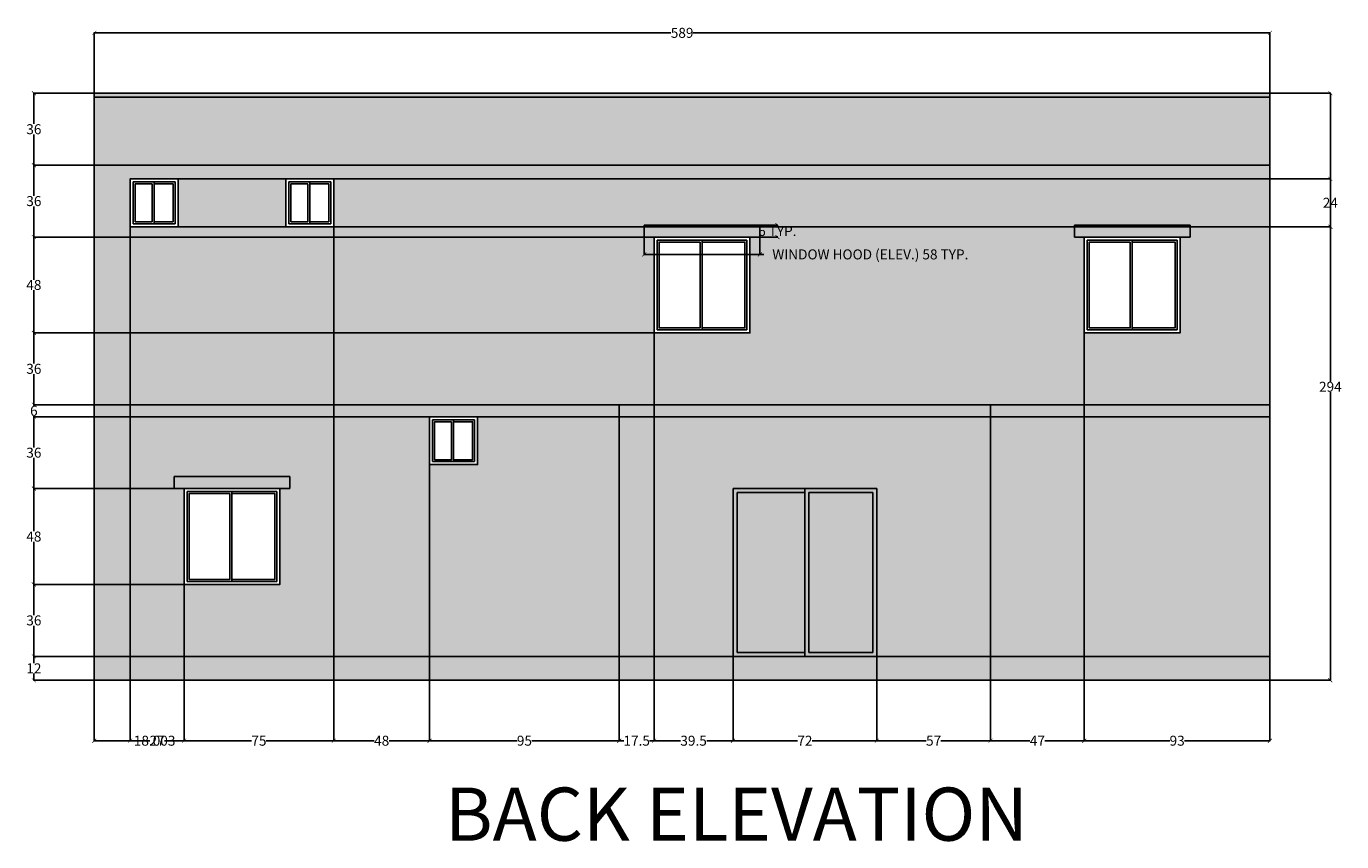
# Model space of a CAD drawing. Units: inches. Extents: x 1455 to 5994, y -182 to 2370.
# Tile 8 of 8: x 5335 to 5994, y -182 to 227. Entities that reach past the tile are written whole.
import ezdxf

# ---------------------------------------------------------------- set-up
doc = ezdxf.new("R2010")
doc.units = ezdxf.units.IN
doc.header["$MEASUREMENT"] = 0
for name, color, linetype, lineweight in [('A-ANNO-DIMS', 2, 'Continuous', 18), ('A-ANNO-TEXT', 7, 'Continuous', 25), ('A-ELEV', 7, 'Continuous', 25), ('A-ELEV-PATT', 8, 'Continuous', 13)]:
    doc.layers.add(name, color=color, linetype=linetype, lineweight=lineweight)
doc.styles.get("Standard").update_dxf_attribs({"font": 'arial.ttf'})
doc.dimstyles.get("Standard").update_dxf_attribs({"dimtxt": 5, "dimasz": 2, "dimexe": 0.18, "dimexo": 0.0625, "dimgap": 0.09, "dimtad": 0, "dimtih": 1, "dimtoh": 1, "dimdec": 1, "dimzin": 0, "dimdsep": 46, "dimlunit": 3, "dimtxsty": 'Standard', "dimblk": 'ARCHTICK', "dimcen": 0.09, "dimadec": 0, "dimazin": 0, "dimtfac": 1, "dimtdec": 1, "dimtofl": 0, "dimtmove": 0, "dimatfit": 3, "dimfxl": 1, "dimtolj": 1, "dimtzin": 0, "dimarcsym": 0})

# ---------------------------------------------------------------- blocks, each defined once
blk = doc.blocks.new('*U8')
for p, q in [((1.5, 1.5), (1.5, 46.5)), ((1.5, 46.5), (24, 46.5)), ((24, 1.5), (24, 46.5)), ((24, 46.5), (46.5, 46.5)), ((46.5, 46.5), (46.5, 1.5)), ((24, 1.5), (1.5, 1.5)), ((46.5, 1.5), (24, 1.5))]:
    blk.add_line(p, q)
blk.add_lwpolyline([(0, 0), (0, 48), (48, 48), (48, 0)], close=True)
for points in [[(23, 45.5), (23, 2.5), (2.5, 2.5), (2.5, 45.5), (23, 45.5)], [(24, 45.5), (45.5, 45.5), (45.5, 2.5), (24, 2.5)]]:
    blk.add_lwpolyline(points)
blk = doc.blocks.new('*U13')
for p, q in [((1.5, 1.5), (1.5, 22.5)), ((1.5, 22.5), (12, 22.5)), ((12, 1.5), (12, 22.5)), ((12, 22.5), (22.5, 22.5)), ((22.5, 22.5), (22.5, 1.5)), ((12, 1.5), (1.5, 1.5)), ((22.5, 1.5), (12, 1.5))]:
    blk.add_line(p, q)
blk.add_lwpolyline([(0, 0), (0, 24), (24, 24), (24, 0)], close=True)
for points in [[(11, 21.5), (11, 2.5), (2.5, 2.5), (2.5, 21.5), (11, 21.5)], [(12, 21.5), (21.5, 21.5), (21.5, 2.5), (12, 2.5)]]:
    blk.add_lwpolyline(points)
blk = doc.blocks.new('WIN-HOOD-ELEV')
for p, q in [((0, 0), (0, 6)), ((0, 6), (58, 6)), ((58, 0), (58, 6)), ((5, 0), (0, 0)), ((53, 0), (58, 0))]:
    blk.add_line(p, q)
blk = doc.blocks.new('_ArchTick')
at = {"color": 0, "linetype": 'ByBlock', "const_width": 0.15}
blk.add_lwpolyline([(-0.5, -0.5), (0.5, 0.5)], dxfattribs=at)
blk = doc.blocks.new('*D33')
at = {"layer": 'A-ANNO-DIMS', "color": 0, "lineweight": -2, "transparency": 16777216}
for p, q in [((5644.62, 121.03), (5644.62, 112.22)), ((5702.62, 121.03), (5702.62, 112.22)), ((5644.62, 112.4), (5702.62, 112.4)), ((5702.62, 112.4), (5704.62, 112.4))]:
    blk.add_line(p, q, dxfattribs=at)
at = {"layer": 'Defpoints', "color": 0, "lineweight": 25, "transparency": 16777216}
for p in [(5644.62, 121.1), (5702.62, 121.1), (5702.62, 112.4)]:
    blk.add_point(p, dxfattribs=at)
at = {"layer": 'A-ANNO-DIMS', "color": 0, "lineweight": -2, "transparency": 16777216, "xscale": 2, "yscale": 2, "zscale": 2, "rotation": 180}
blk.add_blockref('_ArchTick', (5644.62, 112.4), dxfattribs=at)
at = {"layer": 'A-ANNO-DIMS', "color": 0, "lineweight": -2, "transparency": 16777216, "xscale": 2, "yscale": 2, "zscale": 2}
blk.add_blockref('_ArchTick', (5702.62, 112.4), dxfattribs=at)
at = {"layer": 'A-ANNO-DIMS', "color": 0, "transparency": 16777216, "insert": (5757.92, 112.4), "char_height": 5, "attachment_point": 5}
blk.add_mtext('\\A1;WINDOW HOOD (ELEV.) 58 TYP.', dxfattribs=at)
blk = doc.blocks.new('*D34')
at = {"layer": 'A-ANNO-DIMS', "color": 0, "lineweight": -2, "transparency": 16777216}
for p, q in [((5702.68, 127.1), (5711.5, 127.1)), ((5711.32, 127.1), (5711.32, 126.74)), ((5702.68, 121.1), (5711.5, 121.1)), ((5711.32, 121.1), (5711.32, 121.45))]:
    blk.add_line(p, q, dxfattribs=at)
at = {"layer": 'Defpoints', "color": 0, "lineweight": 25, "transparency": 16777216}
for p in [(5702.62, 127.1), (5711.32, 127.1), (5702.62, 121.1)]:
    blk.add_point(p, dxfattribs=at)
at = {"layer": 'A-ANNO-DIMS', "color": 0, "lineweight": -2, "transparency": 16777216, "xscale": 2, "yscale": 2, "zscale": 2}
for p, rotation in [((5711.32, 127.1), 90), ((5711.32, 121.1), 270)]:
    blk.add_blockref('_ArchTick', p, dxfattribs=dict(at, rotation=rotation))
at = {"layer": 'A-ANNO-DIMS', "color": 0, "transparency": 16777216, "insert": (5711.32, 124.1), "char_height": 5, "attachment_point": 5}
blk.add_mtext('\\A1;6 TYP.', dxfattribs=at)
blk = doc.blocks.new('*D117')
at = {"layer": 'A-ANNO-DIMS', "color": 0, "lineweight": -2, "transparency": 16777216}
for p, q in [((5369.12, 193.16), (5369.12, 223.53)), ((5369.12, 223.35), (5658, 223.35)), ((5958.12, 223.35), (5669.24, 223.35)), ((5958.12, 193.16), (5958.12, 223.53))]:
    blk.add_line(p, q, dxfattribs=at)
at = {"layer": 'Defpoints', "color": 0, "lineweight": 25, "transparency": 16777216}
for p in [(5958.12, 223.35), (5369.12, 193.1), (5958.12, 193.1)]:
    blk.add_point(p, dxfattribs=at)
at = {"layer": 'A-ANNO-DIMS', "color": 0, "lineweight": -2, "transparency": 16777216, "xscale": 2, "yscale": 2, "zscale": 2, "rotation": 180}
blk.add_blockref('_ArchTick', (5369.12, 223.35), dxfattribs=at)
at = {"layer": 'A-ANNO-DIMS', "color": 0, "lineweight": -2, "transparency": 16777216, "xscale": 2, "yscale": 2, "zscale": 2}
blk.add_blockref('_ArchTick', (5958.12, 223.35), dxfattribs=at)
at = {"layer": 'A-ANNO-DIMS', "color": 0, "transparency": 16777216, "insert": (5663.62, 223.35), "char_height": 5, "attachment_point": 5}
blk.add_mtext('\\A1;589', dxfattribs=at)
blk = doc.blocks.new('*D118')
at = {"layer": 'A-ANNO-DIMS', "color": 0, "lineweight": -2, "transparency": 16777216}
for p, q in [((5958.18, 193.1), (5988.55, 193.1)), ((5988.37, 193.1), (5988.37, 48.74)), ((5988.37, -100.9), (5988.37, 43.45)), ((5958.18, -100.9), (5988.55, -100.9))]:
    blk.add_line(p, q, dxfattribs=at)
at = {"layer": 'Defpoints', "color": 0, "lineweight": 25, "transparency": 16777216}
for p in [(5958.12, 193.1), (5988.37, 193.1), (5958.12, -100.9)]:
    blk.add_point(p, dxfattribs=at)
at = {"layer": 'A-ANNO-DIMS', "color": 0, "lineweight": -2, "transparency": 16777216, "xscale": 2, "yscale": 2, "zscale": 2}
for p, rotation in [((5988.37, 193.1), 90), ((5988.37, -100.9), 270)]:
    blk.add_blockref('_ArchTick', p, dxfattribs=dict(at, rotation=rotation))
at = {"layer": 'A-ANNO-DIMS', "color": 0, "transparency": 16777216, "insert": (5988.37, 46.1), "char_height": 5, "attachment_point": 5}
blk.add_mtext('\\A1;294', dxfattribs=at)
blk = doc.blocks.new('*D119')
at = {"layer": 'A-ANNO-DIMS', "color": 0, "lineweight": -2, "transparency": 16777216}
for p, q in [((5387.12, 126.2), (5387.12, -131.33)), ((5369.12, -100.97), (5369.12, -131.33)), ((5369.12, -131.15), (5387.12, -131.15)), ((5387.12, -131.15), (5389.12, -131.15))]:
    blk.add_line(p, q, dxfattribs=at)
at = {"layer": 'Defpoints', "color": 0, "lineweight": 25, "transparency": 16777216}
for p in [(5387.12, 126.26), (5369.12, -100.9), (5387.12, -131.15)]:
    blk.add_point(p, dxfattribs=at)
at = {"layer": 'A-ANNO-DIMS', "color": 0, "lineweight": -2, "transparency": 16777216, "xscale": 2, "yscale": 2, "zscale": 2, "rotation": 180}
blk.add_blockref('_ArchTick', (5369.12, -131.15), dxfattribs=at)
at = {"layer": 'A-ANNO-DIMS', "color": 0, "lineweight": -2, "transparency": 16777216, "xscale": 2, "yscale": 2, "zscale": 2}
blk.add_blockref('_ArchTick', (5387.12, -131.15), dxfattribs=at)
at = {"layer": 'A-ANNO-DIMS', "color": 0, "transparency": 16777216, "insert": (5399.36, -131.15), "char_height": 5, "attachment_point": 5}
blk.add_mtext('\\A1;18.003', dxfattribs=at)
blk = doc.blocks.new('*D120')
at = {"layer": 'A-ANNO-DIMS', "color": 0, "lineweight": -2, "transparency": 16777216}
for p, q in [((5387.12, 126.2), (5387.12, -131.33)), ((5414.12, -52.97), (5414.12, -131.33)), ((5387.12, -131.15), (5396.91, -131.15)), ((5414.12, -131.15), (5404.34, -131.15))]:
    blk.add_line(p, q, dxfattribs=at)
at = {"layer": 'Defpoints', "color": 0, "lineweight": 25, "transparency": 16777216}
for p in [(5387.12, 126.26), (5414.12, -52.9), (5414.12, -131.15)]:
    blk.add_point(p, dxfattribs=at)
at = {"layer": 'A-ANNO-DIMS', "color": 0, "lineweight": -2, "transparency": 16777216, "xscale": 2, "yscale": 2, "zscale": 2, "rotation": 180}
blk.add_blockref('_ArchTick', (5387.12, -131.15), dxfattribs=at)
at = {"layer": 'A-ANNO-DIMS', "color": 0, "lineweight": -2, "transparency": 16777216, "xscale": 2, "yscale": 2, "zscale": 2}
blk.add_blockref('_ArchTick', (5414.12, -131.15), dxfattribs=at)
at = {"layer": 'A-ANNO-DIMS', "color": 0, "transparency": 16777216, "insert": (5400.62, -131.15), "char_height": 5, "attachment_point": 5}
blk.add_mtext('\\A1;27', dxfattribs=at)
blk = doc.blocks.new('*D121')
at = {"layer": 'A-ANNO-DIMS', "color": 0, "lineweight": -2, "transparency": 16777216}
for p, q in [((5489.12, 126.2), (5489.12, -131.33)), ((5414.12, -52.97), (5414.12, -131.33)), ((5414.12, -131.15), (5447.95, -131.15)), ((5489.12, -131.15), (5455.29, -131.15))]:
    blk.add_line(p, q, dxfattribs=at)
at = {"layer": 'Defpoints', "color": 0, "lineweight": 25, "transparency": 16777216}
for p in [(5489.12, 126.26), (5414.12, -52.9), (5489.12, -131.15)]:
    blk.add_point(p, dxfattribs=at)
at = {"layer": 'A-ANNO-DIMS', "color": 0, "lineweight": -2, "transparency": 16777216, "xscale": 2, "yscale": 2, "zscale": 2, "rotation": 180}
blk.add_blockref('_ArchTick', (5414.12, -131.15), dxfattribs=at)
at = {"layer": 'A-ANNO-DIMS', "color": 0, "lineweight": -2, "transparency": 16777216, "xscale": 2, "yscale": 2, "zscale": 2}
blk.add_blockref('_ArchTick', (5489.12, -131.15), dxfattribs=at)
at = {"layer": 'A-ANNO-DIMS', "color": 0, "transparency": 16777216, "insert": (5451.62, -131.15), "char_height": 5, "attachment_point": 5}
blk.add_mtext('\\A1;75', dxfattribs=at)
blk = doc.blocks.new('*D122')
at = {"layer": 'A-ANNO-DIMS', "color": 0, "lineweight": -2, "transparency": 16777216}
for p, q in [((5489.12, 126.2), (5489.12, -131.33)), ((5537.12, 7.03), (5537.12, -131.33)), ((5489.12, -131.15), (5509.34, -131.15)), ((5537.12, -131.15), (5516.9, -131.15))]:
    blk.add_line(p, q, dxfattribs=at)
at = {"layer": 'Defpoints', "color": 0, "lineweight": 25, "transparency": 16777216}
for p in [(5489.12, 126.26), (5537.12, 7.1), (5537.12, -131.15)]:
    blk.add_point(p, dxfattribs=at)
at = {"layer": 'A-ANNO-DIMS', "color": 0, "lineweight": -2, "transparency": 16777216, "xscale": 2, "yscale": 2, "zscale": 2, "rotation": 180}
blk.add_blockref('_ArchTick', (5489.12, -131.15), dxfattribs=at)
at = {"layer": 'A-ANNO-DIMS', "color": 0, "lineweight": -2, "transparency": 16777216, "xscale": 2, "yscale": 2, "zscale": 2}
blk.add_blockref('_ArchTick', (5537.12, -131.15), dxfattribs=at)
at = {"layer": 'A-ANNO-DIMS', "color": 0, "transparency": 16777216, "insert": (5513.12, -131.15), "char_height": 5, "attachment_point": 5}
blk.add_mtext('\\A1;48', dxfattribs=at)
blk = doc.blocks.new('*D123')
at = {"layer": 'A-ANNO-DIMS', "color": 0, "lineweight": -2, "transparency": 16777216}
for p, q in [((5537.12, 7.03), (5537.12, -131.33)), ((5632.12, -88.97), (5632.12, -131.33)), ((5537.12, -131.15), (5580.93, -131.15)), ((5632.12, -131.15), (5588.31, -131.15))]:
    blk.add_line(p, q, dxfattribs=at)
at = {"layer": 'Defpoints', "color": 0, "lineweight": 25, "transparency": 16777216}
for p in [(5537.12, 7.1), (5632.12, -88.9), (5632.12, -131.15)]:
    blk.add_point(p, dxfattribs=at)
at = {"layer": 'A-ANNO-DIMS', "color": 0, "lineweight": -2, "transparency": 16777216, "xscale": 2, "yscale": 2, "zscale": 2, "rotation": 180}
blk.add_blockref('_ArchTick', (5537.12, -131.15), dxfattribs=at)
at = {"layer": 'A-ANNO-DIMS', "color": 0, "lineweight": -2, "transparency": 16777216, "xscale": 2, "yscale": 2, "zscale": 2}
blk.add_blockref('_ArchTick', (5632.12, -131.15), dxfattribs=at)
at = {"layer": 'A-ANNO-DIMS', "color": 0, "transparency": 16777216, "insert": (5584.62, -131.15), "char_height": 5, "attachment_point": 5}
blk.add_mtext('\\A1;95', dxfattribs=at)
blk = doc.blocks.new('*D124')
at = {"layer": 'A-ANNO-DIMS', "color": 0, "lineweight": -2, "transparency": 16777216}
for p, q in [((5649.62, 73.03), (5649.62, -131.33)), ((5632.12, -88.97), (5632.12, -131.33)), ((5632.12, -131.15), (5634.5, -131.15)), ((5649.62, -131.15), (5647.24, -131.15))]:
    blk.add_line(p, q, dxfattribs=at)
at = {"layer": 'Defpoints', "color": 0, "lineweight": 25, "transparency": 16777216}
for p in [(5649.62, 73.1), (5632.12, -88.9), (5649.62, -131.15)]:
    blk.add_point(p, dxfattribs=at)
at = {"layer": 'A-ANNO-DIMS', "color": 0, "lineweight": -2, "transparency": 16777216, "xscale": 2, "yscale": 2, "zscale": 2, "rotation": 180}
blk.add_blockref('_ArchTick', (5632.12, -131.15), dxfattribs=at)
at = {"layer": 'A-ANNO-DIMS', "color": 0, "lineweight": -2, "transparency": 16777216, "xscale": 2, "yscale": 2, "zscale": 2}
blk.add_blockref('_ArchTick', (5649.62, -131.15), dxfattribs=at)
at = {"layer": 'A-ANNO-DIMS', "color": 0, "transparency": 16777216, "insert": (5640.87, -131.15), "char_height": 5, "attachment_point": 5}
blk.add_mtext('\\A1;17.5', dxfattribs=at)
blk = doc.blocks.new('*D125')
at = {"layer": 'A-ANNO-DIMS', "color": 0, "lineweight": -2, "transparency": 16777216}
for p, q in [((5649.62, 73.03), (5649.62, -131.33)), ((5689.12, -88.97), (5689.12, -131.33)), ((5649.62, -131.15), (5662.77, -131.15)), ((5689.12, -131.15), (5675.97, -131.15))]:
    blk.add_line(p, q, dxfattribs=at)
at = {"layer": 'Defpoints', "color": 0, "lineweight": 25, "transparency": 16777216}
for p in [(5649.62, 73.1), (5689.12, -88.9), (5689.12, -131.15)]:
    blk.add_point(p, dxfattribs=at)
at = {"layer": 'A-ANNO-DIMS', "color": 0, "lineweight": -2, "transparency": 16777216, "xscale": 2, "yscale": 2, "zscale": 2, "rotation": 180}
blk.add_blockref('_ArchTick', (5649.62, -131.15), dxfattribs=at)
at = {"layer": 'A-ANNO-DIMS', "color": 0, "lineweight": -2, "transparency": 16777216, "xscale": 2, "yscale": 2, "zscale": 2}
blk.add_blockref('_ArchTick', (5689.12, -131.15), dxfattribs=at)
at = {"layer": 'A-ANNO-DIMS', "color": 0, "transparency": 16777216, "insert": (5669.37, -131.15), "char_height": 5, "attachment_point": 5}
blk.add_mtext('\\A1;39.5', dxfattribs=at)
blk = doc.blocks.new('*D126')
at = {"layer": 'A-ANNO-DIMS', "color": 0, "lineweight": -2, "transparency": 16777216}
for p, q in [((5689.12, -88.97), (5689.12, -131.33)), ((5761.12, -88.97), (5761.12, -131.33)), ((5689.12, -131.15), (5721.49, -131.15)), ((5761.12, -131.15), (5728.75, -131.15))]:
    blk.add_line(p, q, dxfattribs=at)
at = {"layer": 'Defpoints', "color": 0, "lineweight": 25, "transparency": 16777216}
for p in [(5689.12, -88.9), (5761.12, -88.9), (5761.12, -131.15)]:
    blk.add_point(p, dxfattribs=at)
at = {"layer": 'A-ANNO-DIMS', "color": 0, "lineweight": -2, "transparency": 16777216, "xscale": 2, "yscale": 2, "zscale": 2, "rotation": 180}
blk.add_blockref('_ArchTick', (5689.12, -131.15), dxfattribs=at)
at = {"layer": 'A-ANNO-DIMS', "color": 0, "lineweight": -2, "transparency": 16777216, "xscale": 2, "yscale": 2, "zscale": 2}
blk.add_blockref('_ArchTick', (5761.12, -131.15), dxfattribs=at)
at = {"layer": 'A-ANNO-DIMS', "color": 0, "transparency": 16777216, "insert": (5725.12, -131.15), "char_height": 5, "attachment_point": 5}
blk.add_mtext('\\A1;72', dxfattribs=at)
blk = doc.blocks.new('*D127')
at = {"layer": 'A-ANNO-DIMS', "color": 0, "lineweight": -2, "transparency": 16777216}
for p, q in [((5761.12, -88.97), (5761.12, -131.33)), ((5818.12, -88.97), (5818.12, -131.33)), ((5761.12, -131.15), (5785.95, -131.15)), ((5818.12, -131.15), (5793.29, -131.15))]:
    blk.add_line(p, q, dxfattribs=at)
at = {"layer": 'Defpoints', "color": 0, "lineweight": 25, "transparency": 16777216}
for p in [(5761.12, -88.9), (5818.12, -88.9), (5818.12, -131.15)]:
    blk.add_point(p, dxfattribs=at)
at = {"layer": 'A-ANNO-DIMS', "color": 0, "lineweight": -2, "transparency": 16777216, "xscale": 2, "yscale": 2, "zscale": 2, "rotation": 180}
blk.add_blockref('_ArchTick', (5761.12, -131.15), dxfattribs=at)
at = {"layer": 'A-ANNO-DIMS', "color": 0, "lineweight": -2, "transparency": 16777216, "xscale": 2, "yscale": 2, "zscale": 2}
blk.add_blockref('_ArchTick', (5818.12, -131.15), dxfattribs=at)
at = {"layer": 'A-ANNO-DIMS', "color": 0, "transparency": 16777216, "insert": (5789.62, -131.15), "char_height": 5, "attachment_point": 5}
blk.add_mtext('\\A1;57', dxfattribs=at)
blk = doc.blocks.new('*D128')
at = {"layer": 'A-ANNO-DIMS', "color": 0, "lineweight": -2, "transparency": 16777216}
for p, q in [((5865.12, 73.03), (5865.12, -131.33)), ((5818.12, -88.97), (5818.12, -131.33)), ((5818.12, -131.15), (5837.85, -131.15)), ((5865.12, -131.15), (5845.39, -131.15))]:
    blk.add_line(p, q, dxfattribs=at)
at = {"layer": 'Defpoints', "color": 0, "lineweight": 25, "transparency": 16777216}
for p in [(5865.12, 73.1), (5818.12, -88.9), (5865.12, -131.15)]:
    blk.add_point(p, dxfattribs=at)
at = {"layer": 'A-ANNO-DIMS', "color": 0, "lineweight": -2, "transparency": 16777216, "xscale": 2, "yscale": 2, "zscale": 2, "rotation": 180}
blk.add_blockref('_ArchTick', (5818.12, -131.15), dxfattribs=at)
at = {"layer": 'A-ANNO-DIMS', "color": 0, "lineweight": -2, "transparency": 16777216, "xscale": 2, "yscale": 2, "zscale": 2}
blk.add_blockref('_ArchTick', (5865.12, -131.15), dxfattribs=at)
at = {"layer": 'A-ANNO-DIMS', "color": 0, "transparency": 16777216, "insert": (5841.62, -131.15), "char_height": 5, "attachment_point": 5}
blk.add_mtext('\\A1;47', dxfattribs=at)
blk = doc.blocks.new('*D129')
at = {"layer": 'A-ANNO-DIMS', "color": 0, "lineweight": -2, "transparency": 16777216}
for p, q in [((5865.12, 73.03), (5865.12, -131.33)), ((5958.12, -100.97), (5958.12, -131.33)), ((5865.12, -131.15), (5907.95, -131.15)), ((5958.12, -131.15), (5915.29, -131.15))]:
    blk.add_line(p, q, dxfattribs=at)
at = {"layer": 'Defpoints', "color": 0, "lineweight": 25, "transparency": 16777216}
for p in [(5865.12, 73.1), (5958.12, -100.9), (5958.12, -131.15)]:
    blk.add_point(p, dxfattribs=at)
at = {"layer": 'A-ANNO-DIMS', "color": 0, "lineweight": -2, "transparency": 16777216, "xscale": 2, "yscale": 2, "zscale": 2, "rotation": 180}
blk.add_blockref('_ArchTick', (5865.12, -131.15), dxfattribs=at)
at = {"layer": 'A-ANNO-DIMS', "color": 0, "lineweight": -2, "transparency": 16777216, "xscale": 2, "yscale": 2, "zscale": 2}
blk.add_blockref('_ArchTick', (5958.12, -131.15), dxfattribs=at)
at = {"layer": 'A-ANNO-DIMS', "color": 0, "transparency": 16777216, "insert": (5911.62, -131.15), "char_height": 5, "attachment_point": 5}
blk.add_mtext('\\A1;93', dxfattribs=at)
blk = doc.blocks.new('*D130')
at = {"layer": 'A-ANNO-DIMS', "color": 0, "lineweight": -2, "transparency": 16777216}
for p, q in [((5369.06, -88.9), (5338.69, -88.9)), ((5338.87, -88.9), (5338.87, -92.3)), ((5338.87, -100.9), (5338.87, -97.5)), ((5369.06, -100.9), (5338.69, -100.9))]:
    blk.add_line(p, q, dxfattribs=at)
at = {"layer": 'Defpoints', "color": 0, "lineweight": 25, "transparency": 16777216}
for p in [(5338.87, -88.9), (5369.12, -88.9), (5369.12, -100.9)]:
    blk.add_point(p, dxfattribs=at)
at = {"layer": 'A-ANNO-DIMS', "color": 0, "lineweight": -2, "transparency": 16777216, "xscale": 2, "yscale": 2, "zscale": 2}
for p, rotation in [((5338.87, -88.9), 90), ((5338.87, -100.9), 270)]:
    blk.add_blockref('_ArchTick', p, dxfattribs=dict(at, rotation=rotation))
at = {"layer": 'A-ANNO-DIMS', "color": 0, "transparency": 16777216, "insert": (5338.87, -94.9), "char_height": 5, "attachment_point": 5}
blk.add_mtext('\\A1;12', dxfattribs=at)
blk = doc.blocks.new('*D131')
at = {"layer": 'A-ANNO-DIMS', "color": 0, "lineweight": -2, "transparency": 16777216}
for p, q in [((5414.06, -52.9), (5338.69, -52.9)), ((5338.87, -52.9), (5338.87, -68.26)), ((5338.87, -88.9), (5338.87, -73.55)), ((5369.06, -88.9), (5338.69, -88.9))]:
    blk.add_line(p, q, dxfattribs=at)
at = {"layer": 'Defpoints', "color": 0, "lineweight": 25, "transparency": 16777216}
for p in [(5338.87, -52.9), (5414.12, -52.9), (5369.12, -88.9)]:
    blk.add_point(p, dxfattribs=at)
at = {"layer": 'A-ANNO-DIMS', "color": 0, "lineweight": -2, "transparency": 16777216, "xscale": 2, "yscale": 2, "zscale": 2}
for p, rotation in [((5338.87, -52.9), 90), ((5338.87, -88.9), 270)]:
    blk.add_blockref('_ArchTick', p, dxfattribs=dict(at, rotation=rotation))
at = {"layer": 'A-ANNO-DIMS', "color": 0, "transparency": 16777216, "insert": (5338.87, -70.9), "char_height": 5, "attachment_point": 5}
blk.add_mtext('\\A1;36', dxfattribs=at)
blk = doc.blocks.new('*D132')
at = {"layer": 'A-ANNO-DIMS', "color": 0, "lineweight": -2, "transparency": 16777216}
for p, q in [((5414.06, -4.9), (5338.69, -4.9)), ((5338.87, -4.9), (5338.87, -26.26)), ((5338.87, -52.9), (5338.87, -31.55)), ((5414.06, -52.9), (5338.69, -52.9))]:
    blk.add_line(p, q, dxfattribs=at)
at = {"layer": 'Defpoints', "color": 0, "lineweight": 25, "transparency": 16777216}
for p in [(5338.87, -4.9), (5414.12, -4.9), (5414.12, -52.9)]:
    blk.add_point(p, dxfattribs=at)
at = {"layer": 'A-ANNO-DIMS', "color": 0, "lineweight": -2, "transparency": 16777216, "xscale": 2, "yscale": 2, "zscale": 2}
for p, rotation in [((5338.87, -4.9), 90), ((5338.87, -52.9), 270)]:
    blk.add_blockref('_ArchTick', p, dxfattribs=dict(at, rotation=rotation))
at = {"layer": 'A-ANNO-DIMS', "color": 0, "transparency": 16777216, "insert": (5338.87, -28.9), "char_height": 5, "attachment_point": 5}
blk.add_mtext('\\A1;48', dxfattribs=at)
blk = doc.blocks.new('*D133')
at = {"layer": 'A-ANNO-DIMS', "color": 0, "lineweight": -2, "transparency": 16777216}
for p, q in [((5369.06, 31.1), (5338.69, 31.1)), ((5338.87, 31.1), (5338.87, 15.74)), ((5338.87, -4.9), (5338.87, 10.45)), ((5414.06, -4.9), (5338.69, -4.9))]:
    blk.add_line(p, q, dxfattribs=at)
at = {"layer": 'Defpoints', "color": 0, "lineweight": 25, "transparency": 16777216}
for p in [(5338.87, 31.1), (5369.12, 31.1), (5414.12, -4.9)]:
    blk.add_point(p, dxfattribs=at)
at = {"layer": 'A-ANNO-DIMS', "color": 0, "lineweight": -2, "transparency": 16777216, "xscale": 2, "yscale": 2, "zscale": 2}
for p, rotation in [((5338.87, 31.1), 90), ((5338.87, -4.9), 270)]:
    blk.add_blockref('_ArchTick', p, dxfattribs=dict(at, rotation=rotation))
at = {"layer": 'A-ANNO-DIMS', "color": 0, "transparency": 16777216, "insert": (5338.87, 13.1), "char_height": 5, "attachment_point": 5}
blk.add_mtext('\\A1;36', dxfattribs=at)
blk = doc.blocks.new('*D134')
at = {"layer": 'A-ANNO-DIMS', "color": 0, "lineweight": -2, "transparency": 16777216}
for p, q in [((5369.06, 37.1), (5338.69, 37.1)), ((5338.87, 37.1), (5338.87, 36.74)), ((5369.06, 31.1), (5338.69, 31.1)), ((5338.87, 31.1), (5338.87, 31.45))]:
    blk.add_line(p, q, dxfattribs=at)
at = {"layer": 'Defpoints', "color": 0, "lineweight": 25, "transparency": 16777216}
for p in [(5338.87, 37.1), (5369.12, 37.1), (5369.12, 31.1)]:
    blk.add_point(p, dxfattribs=at)
at = {"layer": 'A-ANNO-DIMS', "color": 0, "lineweight": -2, "transparency": 16777216, "xscale": 2, "yscale": 2, "zscale": 2}
for p, rotation in [((5338.87, 37.1), 90), ((5338.87, 31.1), 270)]:
    blk.add_blockref('_ArchTick', p, dxfattribs=dict(at, rotation=rotation))
at = {"layer": 'A-ANNO-DIMS', "color": 0, "transparency": 16777216, "insert": (5338.87, 34.1), "char_height": 5, "attachment_point": 5}
blk.add_mtext('\\A1;6', dxfattribs=at)
blk = doc.blocks.new('*D135')
at = {"layer": 'A-ANNO-DIMS', "color": 0, "lineweight": -2, "transparency": 16777216}
for p, q in [((5649.56, 73.1), (5338.69, 73.1)), ((5338.87, 73.1), (5338.87, 57.74)), ((5338.87, 37.1), (5338.87, 52.45)), ((5369.06, 37.1), (5338.69, 37.1))]:
    blk.add_line(p, q, dxfattribs=at)
at = {"layer": 'Defpoints', "color": 0, "lineweight": 25, "transparency": 16777216}
for p in [(5338.87, 73.1), (5649.62, 73.1), (5369.12, 37.1)]:
    blk.add_point(p, dxfattribs=at)
at = {"layer": 'A-ANNO-DIMS', "color": 0, "lineweight": -2, "transparency": 16777216, "xscale": 2, "yscale": 2, "zscale": 2}
for p, rotation in [((5338.87, 73.1), 90), ((5338.87, 37.1), 270)]:
    blk.add_blockref('_ArchTick', p, dxfattribs=dict(at, rotation=rotation))
at = {"layer": 'A-ANNO-DIMS', "color": 0, "transparency": 16777216, "insert": (5338.87, 55.1), "char_height": 5, "attachment_point": 5}
blk.add_mtext('\\A1;36', dxfattribs=at)
blk = doc.blocks.new('*D136')
at = {"layer": 'A-ANNO-DIMS', "color": 0, "lineweight": -2, "transparency": 16777216}
for p, q in [((5649.56, 121.1), (5338.69, 121.1)), ((5338.87, 121.1), (5338.87, 99.74)), ((5338.87, 73.1), (5338.87, 94.45)), ((5649.56, 73.1), (5338.69, 73.1))]:
    blk.add_line(p, q, dxfattribs=at)
at = {"layer": 'Defpoints', "color": 0, "lineweight": 25, "transparency": 16777216}
for p in [(5338.87, 121.1), (5649.62, 121.1), (5649.62, 73.1)]:
    blk.add_point(p, dxfattribs=at)
at = {"layer": 'A-ANNO-DIMS', "color": 0, "lineweight": -2, "transparency": 16777216, "xscale": 2, "yscale": 2, "zscale": 2}
for p, rotation in [((5338.87, 121.1), 90), ((5338.87, 73.1), 270)]:
    blk.add_blockref('_ArchTick', p, dxfattribs=dict(at, rotation=rotation))
at = {"layer": 'A-ANNO-DIMS', "color": 0, "transparency": 16777216, "insert": (5338.87, 97.1), "char_height": 5, "attachment_point": 5}
blk.add_mtext('\\A1;48', dxfattribs=at)
blk = doc.blocks.new('*D137')
at = {"layer": 'A-ANNO-DIMS', "color": 0, "lineweight": -2, "transparency": 16777216}
for p, q in [((5369.06, 157.1), (5338.69, 157.1)), ((5338.87, 157.1), (5338.87, 141.74)), ((5338.87, 121.1), (5338.87, 136.45)), ((5649.56, 121.1), (5338.69, 121.1))]:
    blk.add_line(p, q, dxfattribs=at)
at = {"layer": 'Defpoints', "color": 0, "lineweight": 25, "transparency": 16777216}
for p in [(5338.87, 157.1), (5369.12, 157.1), (5649.62, 121.1)]:
    blk.add_point(p, dxfattribs=at)
at = {"layer": 'A-ANNO-DIMS', "color": 0, "lineweight": -2, "transparency": 16777216, "xscale": 2, "yscale": 2, "zscale": 2}
for p, rotation in [((5338.87, 157.1), 90), ((5338.87, 121.1), 270)]:
    blk.add_blockref('_ArchTick', p, dxfattribs=dict(at, rotation=rotation))
at = {"layer": 'A-ANNO-DIMS', "color": 0, "transparency": 16777216, "insert": (5338.87, 139.1), "char_height": 5, "attachment_point": 5}
blk.add_mtext('\\A1;36', dxfattribs=at)
blk = doc.blocks.new('*D138')
at = {"layer": 'A-ANNO-DIMS', "color": 0, "lineweight": -2, "transparency": 16777216}
for p, q in [((5369.06, 193.1), (5338.69, 193.1)), ((5338.87, 193.1), (5338.87, 177.74)), ((5338.87, 157.1), (5338.87, 172.45)), ((5369.06, 157.1), (5338.69, 157.1))]:
    blk.add_line(p, q, dxfattribs=at)
at = {"layer": 'Defpoints', "color": 0, "lineweight": 25, "transparency": 16777216}
for p in [(5338.87, 193.1), (5369.12, 193.1), (5369.12, 157.1)]:
    blk.add_point(p, dxfattribs=at)
at = {"layer": 'A-ANNO-DIMS', "color": 0, "lineweight": -2, "transparency": 16777216, "xscale": 2, "yscale": 2, "zscale": 2}
for p, rotation in [((5338.87, 193.1), 90), ((5338.87, 157.1), 270)]:
    blk.add_blockref('_ArchTick', p, dxfattribs=dict(at, rotation=rotation))
at = {"layer": 'A-ANNO-DIMS', "color": 0, "transparency": 16777216, "insert": (5338.87, 175.1), "char_height": 5, "attachment_point": 5}
blk.add_mtext('\\A1;36', dxfattribs=at)
blk = doc.blocks.new('*D139')
at = {"layer": 'A-ANNO-DIMS', "color": 0, "lineweight": -2, "transparency": 16777216}
for p, q in [((5411.19, 150.26), (5988.55, 150.26)), ((5988.37, 150.26), (5988.37, 140.86)), ((5988.37, 126.26), (5988.37, 135.66)), ((5411.19, 126.26), (5988.55, 126.26))]:
    blk.add_line(p, q, dxfattribs=at)
at = {"layer": 'Defpoints', "color": 0, "lineweight": 25, "transparency": 16777216}
for p in [(5411.12, 150.26), (5988.37, 150.26), (5411.12, 126.26)]:
    blk.add_point(p, dxfattribs=at)
at = {"layer": 'A-ANNO-DIMS', "color": 0, "lineweight": -2, "transparency": 16777216, "xscale": 2, "yscale": 2, "zscale": 2}
for p, rotation in [((5988.37, 150.26), 90), ((5988.37, 126.26), 270)]:
    blk.add_blockref('_ArchTick', p, dxfattribs=dict(at, rotation=rotation))
at = {"layer": 'A-ANNO-DIMS', "color": 0, "transparency": 16777216, "insert": (5988.37, 138.26), "char_height": 5, "attachment_point": 5}
blk.add_mtext('\\A1;24', dxfattribs=at)

msp = doc.modelspace()

# ---------------------------------------------------------------- hatches: boundary and pattern name
at = {"layer": 'A-ELEV-PATT', "transparency": 33554641}
h = msp.add_hatch(color=256, dxfattribs=at)
h.dxf.hatch_style = 1
h.paths.add_polyline_path([(5958.12, 193.0969), (5369.12, 193.0969), (5369.12, 191.0969), (5958.12, 191.0969)])
h = msp.add_hatch(color=256, dxfattribs=at)
h.dxf.hatch_style = 1
h.paths.add_polyline_path([(5958.12, 191.0969), (5369.12, 191.0969), (5369.12, 157.0969), (5853.12, 157.0969), (5949.12, 157.0969), (5958.12, 157.0969)])
h = msp.add_hatch(color=256, dxfattribs=at)
h.dxf.hatch_style = 1
h.paths.add_polyline_path([(5537.12, 31.0969), (5369.12, 31.0969), (5369.12, -88.9031), (5632.12, -88.9031), (5632.12, 31.0969), (5561.12, 31.0969), (5561.12, 7.0969), (5537.12, 7.0969)])
h.paths.add_polyline_path([(5462.12, 1.0969), (5467.12, 1.0969), (5467.12, -4.9031), (5462.12, -4.9031), (5462.12, -52.9031), (5414.12, -52.9031), (5414.12, -4.9031), (5409.12, -4.9031), (5409.12, 1.0969)], flags=16)
h.paths.add_polyline_path([(5460.62, -6.4031), (5460.62, -51.4031), (5438.12, -51.4031), (5415.62, -51.4031), (5415.62, -6.4031), (5438.12, -6.4031)], flags=0)
h.paths.add_polyline_path([(5459.62, -7.4031), (5459.62, -50.4031), (5438.12, -50.4031), (5438.12, -7.4031)], flags=0)
h.paths.add_polyline_path([(5437.12, -50.4031), (5416.62, -50.4031), (5416.62, -7.4031), (5437.12, -7.4031)], flags=0)
h.paths.add_polyline_path([(5818.12, 31.0969), (5632.12, 31.0969), (5632.12, -88.9031), (5689.12, -88.9031), (5689.12, -4.9031), (5725.12, -4.9031), (5761.12, -4.9031), (5761.12, -88.9031), (5818.12, -88.9031)])
h.paths.add_polyline_path([(5958.12, 31.0969), (5818.12, 31.0969), (5818.12, -88.9031), (5958.12, -88.9031)])
h.paths.add_polyline_path([(5958.12, 157.0969), (5369.12, 157.0969), (5369.12, 37.0969), (5958.12, 37.0969)])
h.paths.add_polyline_path([(5702.62, 121.0969), (5697.62, 121.0969), (5697.62, 73.0969), (5649.62, 73.0969), (5649.62, 121.0969), (5644.62, 121.0969), (5644.62, 127.0969), (5702.62, 127.0969)], flags=16)
h.paths.add_polyline_path([(5696.12, 74.5969), (5673.62, 74.5969), (5651.12, 74.5969), (5651.12, 119.5969), (5673.62, 119.5969), (5696.12, 119.5969)], flags=0)
h.paths.add_polyline_path([(5695.12, 75.5969), (5673.62, 75.5969), (5673.62, 118.5969), (5695.12, 118.5969)], flags=0)
h.paths.add_polyline_path([(5672.62, 75.5969), (5652.12, 75.5969), (5652.12, 118.5969), (5672.62, 118.5969)], flags=0)
h.paths.add_polyline_path([(5860.12, 121.0969), (5860.12, 127.0969), (5918.12, 127.0969), (5918.12, 121.0969), (5913.12, 121.0969), (5913.12, 73.0969), (5865.12, 73.0969), (5865.12, 121.0969)], flags=16)
h.paths.add_polyline_path([(5866.62, 119.5969), (5889.12, 119.5969), (5911.62, 119.5969), (5911.62, 74.5969), (5889.12, 74.5969), (5866.62, 74.5969)], flags=0)
h.paths.add_polyline_path([(5867.62, 118.5969), (5888.12, 118.5969), (5888.12, 75.5969), (5867.62, 75.5969)], flags=0)
h.paths.add_polyline_path([(5889.12, 118.5969), (5910.62, 118.5969), (5910.62, 75.5969), (5889.12, 75.5969)], flags=0)
h.paths.add_polyline_path([(5489.12, 126.2578), (5465.12, 126.2578), (5465.12, 150.2578), (5489.12, 150.2578)], flags=16)
h.paths.add_polyline_path([(5487.62, 127.7578), (5477.12, 127.7578), (5466.62, 127.7578), (5466.62, 148.7578), (5477.12, 148.7578), (5487.62, 148.7578)], flags=0)
h.paths.add_polyline_path([(5486.62, 128.7578), (5477.12, 128.7578), (5477.12, 147.7578), (5486.62, 147.7578)], flags=0)
h.paths.add_polyline_path([(5476.12, 128.7578), (5467.62, 128.7578), (5467.62, 147.7578), (5476.12, 147.7578)], flags=0)
h.paths.add_polyline_path([(5411.1226, 126.2578), (5387.1226, 126.2578), (5387.1226, 150.2578), (5411.1226, 150.2578)], flags=16)
h.paths.add_polyline_path([(5409.6226, 127.7578), (5399.1226, 127.7578), (5388.6226, 127.7578), (5388.6226, 148.7578), (5399.1226, 148.7578), (5409.6226, 148.7578)], flags=0)
h.paths.add_polyline_path([(5408.6226, 128.7578), (5399.1226, 128.7578), (5399.1226, 147.7578), (5408.6226, 147.7578)], flags=0)
h.paths.add_polyline_path([(5398.1226, 128.7578), (5389.6226, 128.7578), (5389.6226, 147.7578), (5398.1226, 147.7578)], flags=0)
h = msp.add_hatch(color=256, dxfattribs=at)
h.dxf.hatch_style = 1
h.paths.add_polyline_path([(5702.62, 127.0969), (5644.62, 127.0969), (5644.62, 121.0969), (5649.62, 121.0969), (5697.62, 121.0969), (5702.62, 121.0969)])
h.paths.add_polyline_path([(5918.12, 127.0969), (5860.12, 127.0969), (5860.12, 121.0969), (5865.12, 121.0969), (5913.12, 121.0969), (5918.12, 121.0969)])
h.paths.add_polyline_path([(5467.12, 1.0969), (5462.12, 1.0969), (5409.12, 1.0969), (5409.12, -4.9031), (5414.12, -4.9031), (5462.12, -4.9031), (5467.12, -4.9031)])
h = msp.add_hatch(color=256, dxfattribs=at)
h.dxf.hatch_style = 1
h.paths.add_polyline_path([(5632.12, 37.0969), (5369.12, 37.0969), (5369.12, 31.0969), (5632.12, 31.0969)])
h.paths.add_polyline_path([(5818.12, 37.0969), (5632.12, 37.0969), (5632.12, 31.0969), (5818.12, 31.0969)])
h.paths.add_polyline_path([(5958.12, 37.0969), (5818.12, 37.0969), (5818.12, 31.0969), (5958.12, 31.0969)])
h = msp.add_hatch(color=256, dxfattribs=at)
h.dxf.hatch_style = 1
h.paths.add_polyline_path([(5725.12, -4.9031), (5689.12, -4.9031), (5689.12, -88.9031), (5725.12, -88.9031), (5725.12, -86.9031), (5691.12, -86.9031), (5691.12, -6.9031), (5725.12, -6.9031)])
h.paths.add_polyline_path([(5761.12, -4.9031), (5725.12, -4.9031), (5725.12, -88.9031), (5761.12, -88.9031)])
h.paths.add_polyline_path([(5727.12, -6.9031), (5759.12, -6.9031), (5759.12, -86.9031), (5727.12, -86.9031)], flags=16)
h = msp.add_hatch(color=256, dxfattribs=at)
h.dxf.hatch_style = 1
h.paths.add_polyline_path([(5725.12, -6.9031), (5691.12, -6.9031), (5691.12, -86.9031), (5725.12, -86.9031)])
h.paths.add_polyline_path([(5759.12, -6.9031), (5727.12, -6.9031), (5727.12, -86.9031), (5759.12, -86.9031)])
h = msp.add_hatch(color=256, dxfattribs=at)
h.dxf.hatch_style = 1
h.paths.add_polyline_path([(5958.12, -88.9031), (5369.12, -88.9031), (5369.12, -100.9031), (5958.12, -100.9031)])

# ---------------------------------------------------------------- linework, layer by layer
at = {"layer": 'A-ELEV'}
for p, q in [((5369.12, 157.0969), (5369.12, 193.0969)), ((5369.12, 193.0969), (5958.12, 193.0969)), ((5958.12, 157.0969), (5958.12, 193.0969)), ((5369.12, 191.0969), (5958.12, 191.0969)), ((5369.12, 157.0969), (5958.12, 157.0969)), ((5369.12, 157.0969), (5369.12, -100.9031)), ((5853.12, 157.0969), (5949.12, 157.0969)), ((5949.12, 157.0969), (5958.12, 157.0969)), ((5958.12, 157.0969), (5958.12, -100.9031)), ((5369.12, -88.9031), (5369.12, 37.0969)), ((5958.12, 37.0969), (5369.12, 37.0969)), ((5369.12, 37.0969), (5958.12, 37.0969)), ((5632.12, -88.9031), (5632.12, 37.0969)), ((5818.12, -88.9031), (5818.12, 37.0969)), ((5958.12, -88.9031), (5958.12, 37.0969)), ((5958.12, 31.0969), (5369.12, 31.0969)), ((5409.12, -4.9031), (5409.12, 1.0969)), ((5409.12, 1.0969), (5462.12, 1.0969)), ((5462.12, 1.0969), (5467.12, 1.0969)), ((5467.12, 1.0969), (5467.12, -4.9031)), ((5414.12, -4.9031), (5409.12, -4.9031)), ((5467.12, -4.9031), (5462.12, -4.9031)), ((5689.12, -4.9031), (5725.12, -4.9031)), ((5689.12, -88.9031), (5689.12, -4.9031)), ((5725.12, -4.9031), (5725.12, -88.9031)), ((5725.12, -4.9031), (5761.12, -4.9031)), ((5725.12, -88.9031), (5725.12, -4.9031)), ((5761.12, -4.9031), (5761.12, -88.9031)), ((5691.12, -6.9031), (5725.12, -6.9031)), ((5691.12, -86.9031), (5691.12, -6.9031)), ((5727.12, -6.9031), (5759.12, -6.9031)), ((5727.12, -86.9031), (5727.12, -6.9031)), ((5759.12, -6.9031), (5759.12, -86.9031)), ((5958.12, -88.9031), (5369.12, -88.9031)), ((5369.12, -100.9031), (5369.12, -88.9031)), ((5725.12, -88.9031), (5689.12, -88.9031)), ((5725.12, -86.9031), (5691.12, -86.9031)), ((5761.12, -88.9031), (5725.12, -88.9031)), ((5759.12, -86.9031), (5727.12, -86.9031)), ((5958.12, -100.9031), (5958.12, -88.9031)), ((5958.12, -100.9031), (5369.12, -100.9031))]:
    msp.add_line(p, q, dxfattribs=at)

# ---------------------------------------------------------------- block references
for name, p in [('*U13', (5387.1226, 126.2578)), ('*U13', (5465.12, 126.2578)), ('WIN-HOOD-ELEV', (5644.62, 121.097)), ('WIN-HOOD-ELEV', (5860.12, 121.097)), ('*U8', (5649.62, 73.0969)), ('*U8', (5865.12, 73.0969)), ('*U13', (5537.12, 7.0969)), ('*U8', (5414.12, -52.9031))]:
    msp.add_blockref(name, p, dxfattribs=at)

# ---------------------------------------------------------------- texts
at = {"layer": 'A-ANNO-TEXT'}
msp.add_text('BACK ELEVATION', height=26.640459, dxfattribs=at).set_placement((5544.8278, -181.252))

# ---------------------------------------------------------------- dimensions: what is measured, and where the dimension line sits
at = {"layer": 'A-ANNO-DIMS'}
for base, p1, p2, override, picture, middle in [((5958.12, 223.3469), (5369.12, 193.0969), (5958.12, 193.0969), {"dimdec": 0, "dimlfac": 1, "dimrnd": 0, "dimzin": 0, "dimdsep": 46, "dimlunit": 2}, '*D117', (5663.62, 223.3469)), ((5387.1226, -131.1531), (5369.12, -100.9031), (5387.1226, 126.2578), {"dimdec": 3, "dimlfac": 1, "dimrnd": 0, "dimzin": 0, "dimdsep": 46, "dimlunit": 2}, '*D119', (5399.3558, -131.1531)), ((5414.12, -131.1531), (5387.1226, 126.2578), (5414.12, -52.9031), {"dimdec": 0, "dimlfac": 1, "dimrnd": 0, "dimzin": 0, "dimdsep": 46, "dimlunit": 2}, '*D120', (5400.6213, -131.1531)), ((5489.12, -131.1531), (5414.12, -52.9031), (5489.12, 126.2578), {"dimdec": 0, "dimlfac": 1, "dimrnd": 0, "dimzin": 0, "dimdsep": 46, "dimlunit": 2}, '*D121', (5451.62, -131.1531)), ((5537.12, -131.1531), (5489.12, 126.2578), (5537.12, 7.0969), {"dimdec": 0, "dimlfac": 1, "dimrnd": 0, "dimzin": 0, "dimdsep": 46, "dimlunit": 2}, '*D122', (5513.12, -131.1531)), ((5649.62, -131.1531), (5632.12, -88.9031), (5649.62, 73.0969), {"dimdec": 1, "dimlfac": 1, "dimrnd": 0, "dimzin": 0, "dimdsep": 46, "dimlunit": 2}, '*D124', (5640.87, -131.1531)), ((5689.12, -131.1531), (5649.62, 73.0969), (5689.12, -88.9031), {"dimdec": 1, "dimlfac": 1, "dimrnd": 0, "dimzin": 0, "dimdsep": 46, "dimlunit": 2}, '*D125', (5669.37, -131.1531)), ((5865.12, -131.1531), (5818.12, -88.9031), (5865.12, 73.0969), {"dimdec": 0, "dimlfac": 1, "dimrnd": 0, "dimzin": 0, "dimdsep": 46, "dimlunit": 2}, '*D128', (5841.62, -131.1531)), ((5958.12, -131.1531), (5865.12, 73.0969), (5958.12, -100.9031), {"dimdec": 0, "dimlfac": 1, "dimrnd": 0, "dimzin": 0, "dimdsep": 46, "dimlunit": 2}, '*D129', (5911.62, -131.1531)), ((5632.12, -131.1531), (5537.12, 7.0969), (5632.12, -88.9031), {"dimdec": 0, "dimlfac": 1, "dimrnd": 0, "dimzin": 0, "dimdsep": 46, "dimlunit": 2}, '*D123', (5584.62, -131.1531)), ((5761.12, -131.1531), (5689.12, -88.9031), (5761.12, -88.9031), {"dimdec": 0, "dimlfac": 1, "dimrnd": 0, "dimzin": 0, "dimdsep": 46, "dimlunit": 2}, '*D126', (5725.12, -131.1531)), ((5818.12, -131.1531), (5761.12, -88.9031), (5818.12, -88.9031), {"dimdec": 0, "dimlfac": 1, "dimrnd": 0, "dimzin": 0, "dimdsep": 46, "dimlunit": 2}, '*D127', (5789.62, -131.1531))]:
    dim = msp.add_linear_dim(base=base, p1=p1, p2=p2, dimstyle='Standard', override=override, dxfattribs=at)
    dim.commit()
    dim.dimension.update_dxf_attribs({"geometry": picture, "text_midpoint": middle})
for base, p1, p2, picture, middle in [((5338.87, 193.0969), (5369.12, 157.0969), (5369.12, 193.0969), '*D138', (5338.87, 175.0969)), ((5988.37, 193.0969), (5958.12, -100.9031), (5958.12, 193.0969), '*D118', (5988.37, 46.0969)), ((5338.87, 157.0969), (5649.62, 121.0969), (5369.12, 157.0969), '*D137', (5338.87, 139.0969)), ((5988.37, 150.2578), (5411.1226, 126.2578), (5411.1226, 150.2578), '*D139', (5988.37, 138.2578)), ((5338.87, 121.0969), (5649.62, 73.0969), (5649.62, 121.0969), '*D136', (5338.87, 97.0969)), ((5338.87, 73.0969), (5369.12, 37.0969), (5649.62, 73.0969), '*D135', (5338.87, 55.0969)), ((5338.87, 37.0969), (5369.12, 31.0969), (5369.12, 37.0969), '*D134', (5338.87, 34.0969)), ((5338.87, 31.0969), (5414.12, -4.9031), (5369.12, 31.0969), '*D133', (5338.87, 13.0969)), ((5338.87, -4.9031), (5414.12, -52.9031), (5414.12, -4.9031), '*D132', (5338.87, -28.9031)), ((5338.87, -52.9031), (5369.12, -88.9031), (5414.12, -52.9031), '*D131', (5338.87, -70.9031)), ((5338.87, -88.9031), (5369.12, -100.9031), (5369.12, -88.9031), '*D130', (5338.87, -94.9031))]:
    dim = msp.add_linear_dim(base=base, p1=p1, p2=p2, angle=90, dimstyle='Standard', override={"dimdec": 0, "dimlfac": 1, "dimrnd": 0, "dimzin": 0, "dimdsep": 46, "dimlunit": 2}, dxfattribs=at)
    dim.commit()
    dim.dimension.update_dxf_attribs({"geometry": picture, "text_midpoint": middle})
dim = msp.add_linear_dim(base=(5702.62, 112.3969), p1=(5644.62, 121.0969), p2=(5702.62, 121.0969), text='WINDOW HOOD (ELEV.) <> TYP.', dimstyle='Standard', override={"dimdec": 0, "dimlfac": 1, "dimrnd": 0, "dimzin": 0, "dimdsep": 46, "dimlunit": 2}, dxfattribs=at)
dim.commit()
dim.dimension.update_dxf_attribs({"geometry": '*D33', "text_midpoint": (5757.9211, 112.3969)})
dim = msp.add_linear_dim(base=(5711.32, 127.0969), p1=(5702.62, 121.0969), p2=(5702.62, 127.0969), angle=90, text='<> TYP.', dimstyle='Standard', override={"dimdec": 0, "dimlfac": 1, "dimrnd": 0, "dimzin": 0, "dimdsep": 46, "dimlunit": 2}, dxfattribs=at)
dim.commit()
dim.dimension.update_dxf_attribs({"geometry": '*D34', "text_midpoint": (5711.32, 124.0969)})

doc.saveas('drawing.dxf')
